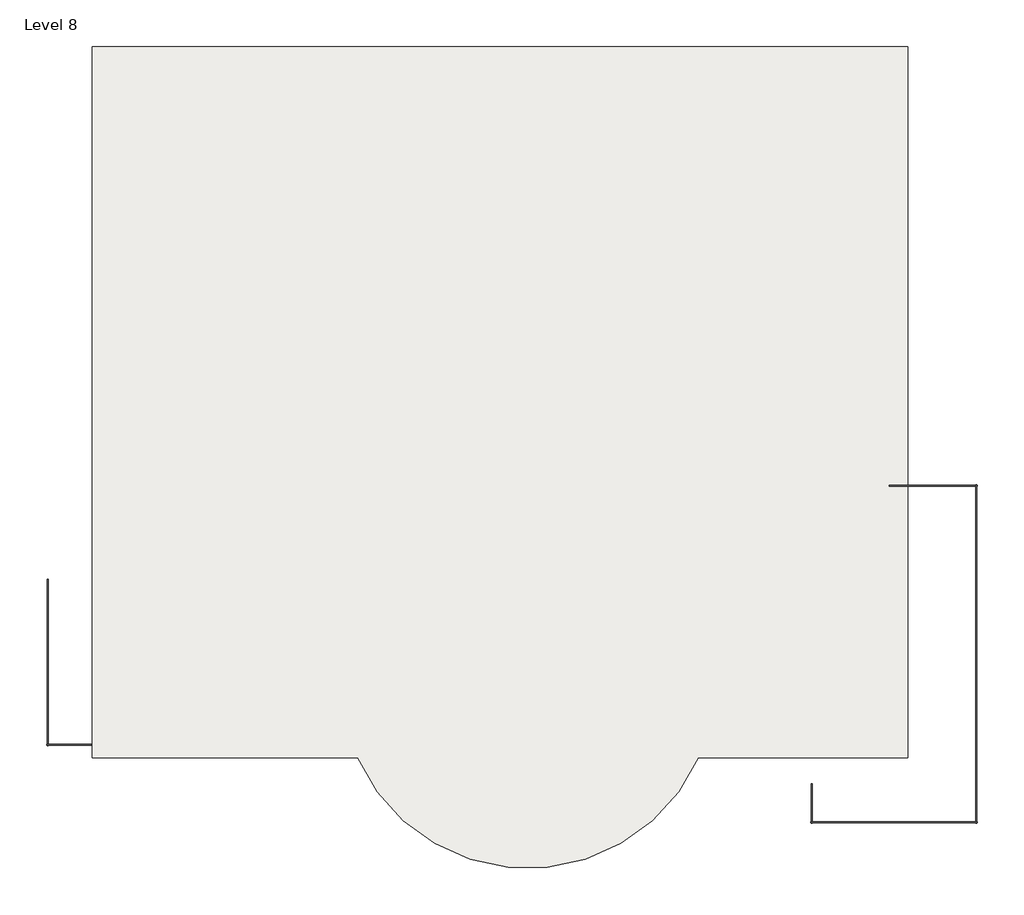
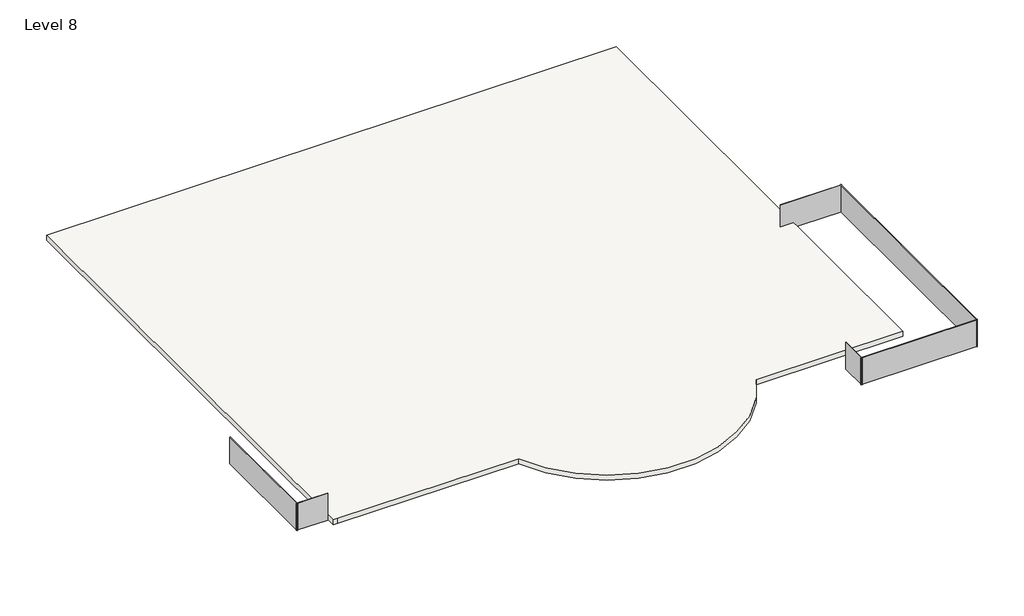
# One storey: 6 plates, 1 slab.
"""IFC4 building model written with IfcOpenShell, lengths in millimetres."""

from ifc_helpers import new_model, si_unit, point, frame, frame_2d, origin, place, context, project, spatial, polyline, circle_curve, trimmed, segment, composite_curve, outline, extrude, transform, mapped, element, save
from components import system_panel_glazed_7d767388, system_panel_glazed_c55d8a5b, system_panel_glazed_a5f349e9, system_panel_glazed_f6fb2dd6, system_panel_glazed_fdc1463f, system_panel_glazed_b99798ed

model = new_model("IFC4")

# Units and contexts
model_context = context("Model", 3, world=origin())
ifc_project = project(units=[si_unit("LENGTHUNIT", "METRE", prefix="MILLI")], contexts=[model_context])

# Site, building, storey
site = spatial("IfcSite", under=ifc_project)
building = spatial("IfcBuilding", under=site)
storey = spatial("IfcBuildingStorey", under=building, Name="Level 8", Elevation=12877.8)

# Plates
placement = place(None, origin())
system_panel_glazed_shape = system_panel_glazed_7d767388(model_context)
element("IfcPlate", 1, ObjectType="System Panel : Glazed", at=placement, inside=storey, context=model_context, shape_type="MappedRepresentation", body=[
    mapped(system_panel_glazed_shape, transform((-17306.4505427, -13712.8739591, 12877.8), x_axis=(1.0, 0.0, 0.0), y_axis=(0.0, 1.0, 0.0), z_axis=(0.0, 0.0, 1.0))),
])
system_panel_glazed_2_shape = system_panel_glazed_c55d8a5b(model_context)
element("IfcPlate", 2, ObjectType="System Panel : Glazed", at=placement, inside=storey, context=model_context, shape_type="MappedRepresentation", body=[
    mapped(system_panel_glazed_2_shape, transform((7558.5964352, -16051.9778294, 12877.8), x_axis=(1.0, 0.0, 0.0), y_axis=(0.0, 1.0, 0.0), z_axis=(0.0, 0.0, 1.0))),
])
system_panel_glazed_3_shape = system_panel_glazed_a5f349e9(model_context)
element("IfcPlate", 3, ObjectType="System Panel : Glazed", at=placement, inside=storey, context=model_context, shape_type="MappedRepresentation", body=[
    mapped(system_panel_glazed_3_shape, transform((-17979.5505427, -11201.4489591, 12877.8), x_axis=(0.0, -1.0, 0.0), y_axis=(1.0, 0.0, 0.0), z_axis=(0.0, 0.0, 1.0))),
])
system_panel_glazed_4_shape = system_panel_glazed_f6fb2dd6(model_context)
element("IfcPlate", 4, ObjectType="System Panel : Glazed", at=placement, inside=storey, context=model_context, shape_type="MappedRepresentation", body=[
    mapped(system_panel_glazed_4_shape, transform((5043.9964352, -15455.0778294, 12877.8), x_axis=(0.0, -1.0, 0.0), y_axis=(1.0, 0.0, 0.0), z_axis=(0.0, 0.0, 1.0))),
])
system_panel_glazed_5_shape = system_panel_glazed_fdc1463f(model_context)
element("IfcPlate", 5, ObjectType="System Panel : Glazed", at=placement, inside=storey, context=model_context, shape_type="MappedRepresentation", body=[
    mapped(system_panel_glazed_5_shape, transform((10073.1964352, -10950.2293258, 12877.8), x_axis=(0.0, 1.0, 0.0), y_axis=(-1.0, 0.0, 0.0), z_axis=(0.0, 0.0, 1.0))),
])
system_panel_glazed_6_shape = system_panel_glazed_b99798ed(model_context)
element("IfcPlate", 6, ObjectType="System Panel : Glazed", at=placement, inside=storey, context=model_context, shape_type="MappedRepresentation", body=[
    mapped(system_panel_glazed_6_shape, transform((8746.8229462, -5848.4808221, 12877.8), x_axis=(-1.0, 0.0, 0.0), y_axis=(0.0, -1.0, 0.0), z_axis=(0.0, 0.0, 1.0))),
])

# Slab
element("IfcSlab", 7, ObjectType="9\"", at=placement, inside=storey, context=model_context, shape_type="SweptSolid", body=[
    extrude(outline(composite_curve([segment(polyline([(-16607.9505427, 7359.5191779), (7979.2494573, 7359.5191779), (7979.2494573, -14078.0808221), (1652.8739931, -14078.0808221)]), True, "CONTINUOUS"), segment(trimmed(circle_curve(frame_2d((-3476.1505427, -11788.3650223)), 5616.9111737), [point((1652.8739931, -14078.0808221))], [point((-8605.1750786, -14078.0808221))], False, "CARTESIAN"), True, "CONTINUOUS"), segment(polyline([(-8605.1750786, -14078.0808221), (-16404.7505427, -14078.0808221), (-16607.9505427, -14078.0808221), (-16607.9505427, 7359.5191779)]), True, "CONTINUOUS")], self_intersect=False)), frame((0.0, 0.0, 12877.8), z_axis=(0.0, 0.0, 1.0), x_axis=(1.0, 0.0, 0.0)), (0.0, 0.0, 1.0), 228.6),
])

save(model, "model.ifc")

# Revit data of these elements
# Type "System Panel : Glazed"
#   Construction Type Id = "GSP4R"
#   Analytic Construction = "1/8 in Pilkington single glazing"
#   Visual Light Transmittance = 0.9
#   Solar Heat Gain Coefficient = 0.86
#   Heat Transfer Coefficient (U) = 1.18115 BTU/(h·ft²·°F)
# Type "9\""
#   Assembly Code = "B1010"
#   Function = 0
#   Layers, outside or top first: 0' - 9" no material (function 1)
# Elements 1, 2, 3, 4, 5, 6 (IfcPlate, "System Panel : Glazed")
#   Phase Created = New Construction
#   Materials on its faces: "Glass"
# Element 7 (IfcSlab, "9\"")
#   built-in parameter 1001955 = 1.5708 (stored number, unit not read)
#   Height Offset From Level = 0' - 9"
#   Phase Created = New Construction
#   Materials on its faces: "Default Floor"
# Materials
#   "Glass": class "Glass", colour RGB 0 128 192, transparency 0.75, Description = "Soda Lime Glass", Cost = 0
#   "Default Floor": colour RGB 128 128 128, transparency 0
